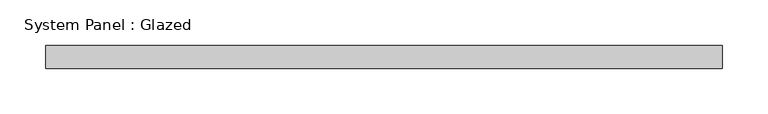
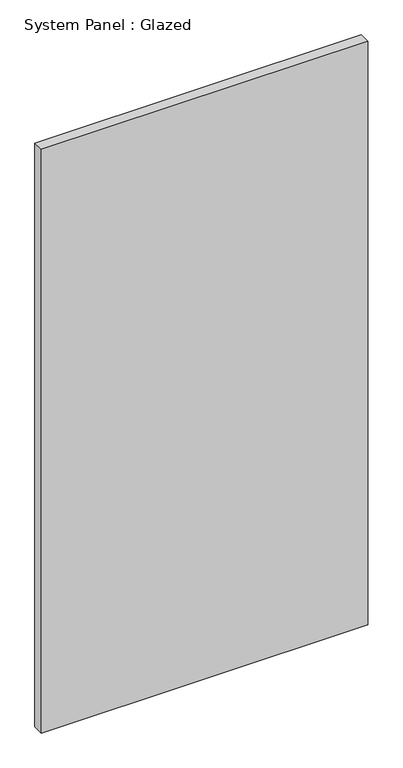
"""IFC4 building model written with IfcOpenShell, lengths in millimetres: plate geometry, System Panel : Glazed."""

from ifc_helpers import new_model, si_unit, origin, origin_with_axes, place, context, project, spatial, polyline, outline, extrude, source, transform, mapped, element, save


def system_panel_glazed_14be1180(model_context):
    return source(origin(), model_context, "Body", "SweptSolid", [
        extrude(outline(polyline([(371.475, 19.05), (-371.475, 19.05), (-371.475, 44.45), (371.475, 44.45), (371.475, 19.05)])), origin_with_axes(), (0.0, 0.0, 1.0), 1404.3368617),
    ])


if __name__ == "__main__":
    model = new_model("IFC4")
    model_context = context("Model", 3, world=origin())
    ifc_project = project(units=[si_unit("LENGTHUNIT", "METRE", prefix="MILLI")], contexts=[model_context])
    site = spatial("IfcSite", under=ifc_project)
    building = spatial("IfcBuilding", under=site)
    placement = place(None, origin())
    system_panel_glazed_shape = system_panel_glazed_14be1180(model_context)
    element("IfcPlate", 1, ObjectType="System Panel : Glazed", at=placement, inside=building, context=model_context, shape_type="MappedRepresentation", body=[
        mapped(system_panel_glazed_shape, transform((0.0, 0.0, 0.0), x_axis=(1.0, 0.0, 0.0), y_axis=(0.0, 1.0, 0.0), z_axis=(0.0, 0.0, 1.0))),
    ])
    save(model, "model.ifc")

# Revit data of these elements
# Type "System Panel : Glazed"
#   Construction Type Id = "GSP4R"
#   Analytic Construction = "1/8 in Pilkington single glazing"
#   Visual Light Transmittance = 0.9
#   Solar Heat Gain Coefficient = 0.86
#   Heat Transfer Coefficient (U) = 1.18115 BTU/(h·ft²·°F)
#   Define Thermal Properties by = 1
# Element 1 (IfcPlate, "System Panel : Glazed")
#   Materials on its faces: "Glass"
# Materials
#   "Glass": class "Glass", colour RGB 0 128 192, transparency 0.75, Description = "Soda Lime Glass", Cost = 0
